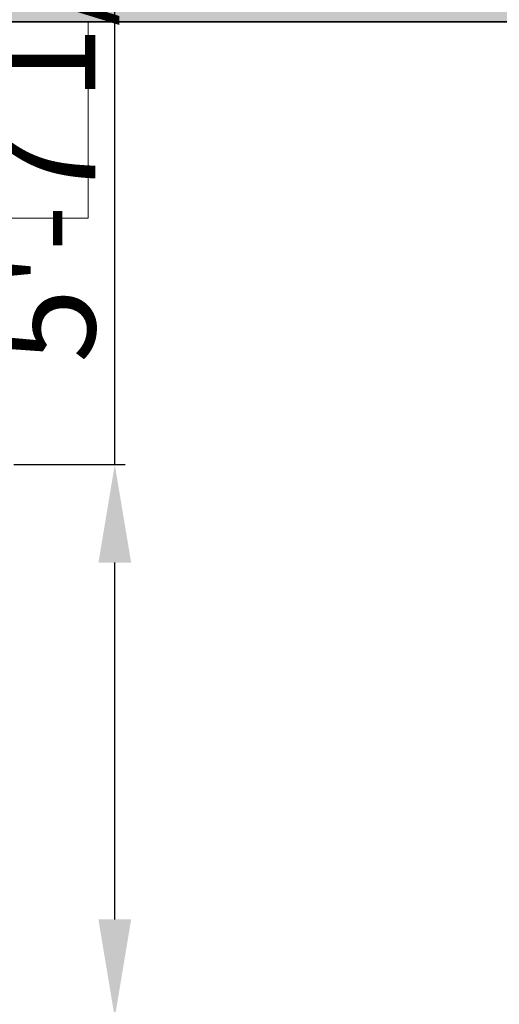
# Model space of a CAD drawing. Units: inches. Extents: x 2083 to 3317, y 1141 to 2115.
# Tile 14 of 256: x 2324 to 2382, y 1296 to 1417. Entities that reach past the tile are written whole.
import ezdxf

# ---------------------------------------------------------------- set-up
doc = ezdxf.new("R2010")
doc.units = ezdxf.units.IN
for name, color, linetype, lineweight in [('A-ANNO-DIMS', 2, 'Continuous', 18), ('A-FLOR-CASE', 8, 'Continuous', 18), ('A-WALL', 7, 'Continuous', 35)]:
    doc.layers.add(name, color=color, linetype=linetype, lineweight=lineweight)
doc.layers.add('A-WALL-PATT', color=251, linetype='Continuous', lineweight=13, true_color=0x636466)
doc.styles.get("Standard").update_dxf_attribs({"font": 'arial.ttf'})
doc.dimstyles.new('ISO-25', dxfattribs={"dimtxt": 12, "dimasz": 12, "dimexe": 1.25, "dimexo": 0.625, "dimtad": 1, "dimlunit": 3, "dimtxsty": 'Standard', "dimcen": 2.5, "dimadec": 0, "dimazin": 0, "dimtfac": 1, "dimtmove": 0, "dimatfit": 3, "dimfxl": 1, "dimarcsym": 0})

# ---------------------------------------------------------------- blocks, each defined once
blk = doc.blocks.new('CASEWORK-96X24')
for q in [(0, 0), (24, 96)]:
    blk.add_line((0, 96), q)
blk = doc.blocks.new('*D23')
at = {"layer": 'A-ANNO-DIMS', "color": 0, "lineweight": -2, "transparency": 16777216}
for p, q in [((2335.21, 1362.11), (2335.21, 1476.47)), ((2322.89, 1362.11), (2336.46, 1362.11)), ((2335.21, 1306.47), (2335.21, 1350.11)), ((2322.89, 1294.47), (2336.46, 1294.47))]:
    blk.add_line(p, q, dxfattribs=at)
at = {"layer": 'A-ANNO-DIMS', "color": 0, "transparency": 16777216}
for points in [[(2333.21, 1350.11), (2337.21, 1350.11), (2335.21, 1362.11)], [(2333.21, 1306.47), (2337.21, 1306.47), (2335.21, 1294.47)]]:
    blk.add_solid(points, dxfattribs=at)
at = {"layer": 'Defpoints', "color": 0, "transparency": 16777216}
for p in [(2322.26, 1362.11), (2335.21, 1362.11), (2322.26, 1294.47)]:
    blk.add_point(p, dxfattribs=at)
at = {"layer": 'A-ANNO-DIMS', "color": 0, "transparency": 16777216, "insert": (2328.38, 1425.29), "char_height": 12, "attachment_point": 5, "rotation": 90}
blk.add_mtext('5\'-7 1/2" TYP.', dxfattribs=at)
blk = doc.blocks.new('*D30')
at = {"layer": 'A-ANNO-DIMS', "color": 0, "lineweight": -2, "transparency": 16777216}
for p, q in [((2240.02, 1445.27), (2240.02, 1448.05)), ((2254.33, 1445.27), (2254.33, 1448.05)), ((2228.02, 1446.8), (2216.02, 1446.8)), ((2240.02, 1446.8), (2254.33, 1446.8)), ((2266.33, 1446.8), (2413.76, 1446.8))]:
    blk.add_line(p, q, dxfattribs=at)
at = {"layer": 'A-ANNO-DIMS', "color": 0, "transparency": 16777216}
for points in [[(2228.02, 1448.8), (2228.02, 1444.8), (2240.02, 1446.8)], [(2266.33, 1448.8), (2266.33, 1444.8), (2254.33, 1446.8)]]:
    blk.add_solid(points, dxfattribs=at)
at = {"layer": 'Defpoints', "color": 0, "transparency": 16777216}
for p in [(2254.33, 1446.8), (2240.02, 1444.65), (2254.33, 1444.65)]:
    blk.add_point(p, dxfattribs=at)
at = {"layer": 'A-ANNO-DIMS', "color": 0, "transparency": 16777216, "insert": (2346.05, 1453.63), "char_height": 12, "attachment_point": 5}
blk.add_mtext('WC 1\'-2 1/2" TYP.', dxfattribs=at)

msp = doc.modelspace()

# ---------------------------------------------------------------- hatches: boundary and pattern name
at = {"layer": 'A-WALL-PATT'}
h = msp.add_hatch(color=256, dxfattribs=at)
h.dxf.hatch_style = 1
h.paths.add_polyline_path([(3126.96, 2020.761), (2748.96, 2020.761), (2604.96, 2020.761), (2226.96, 2020.761), (2226.96, 1702.761), (2466.96, 1702.761), (2466.96, 1582.761), (2418.96, 1582.761), (2418.96, 1477.761), (2226.96, 1477.761), (2226.96, 1263.261), (2544.96, 1263.261), (2544.96, 1411.761), (2604.96, 1411.761), (2685.96, 1411.761), (2685.96, 1420.761), (2604.96, 1420.761), (2604.96, 1573.761), (2604.96, 1702.761), (2604.96, 2011.761), (2748.96, 2011.761), (2748.96, 1702.761), (2862.96, 1702.761), (2862.96, 1621.761), (2871.96, 1621.761), (2871.96, 1702.761), (2883.96, 1702.761), (2883.96, 1706.939, -0.0264593), (2883.96, 1711.761), (2757.96, 1711.761), (2757.96, 1807.761), (2787.96, 1807.761), (2787.96, 1812.261), (2757.96, 1812.261), (2757.96, 2011.761), (2877.96, 2011.761), (2877.96, 1812.261), (2847.96, 1812.261), (2847.96, 1807.761), (2889.836, 1807.761), (2889.836, 1812.261), (2882.46, 1812.261), (2882.46, 2011.761), (3117.96, 2011.761), (3117.96, 1812.261), (2937.836, 1812.261), (2937.836, 1807.761), (2995.71, 1807.761), (2995.71, 1796.118), (3000.21, 1796.118), (3000.21, 1807.761), (3117.96, 1807.761), (3117.96, 1711.761), (3000.21, 1711.761), (3000.21, 1760.118), (2998.573, 1760.118, -0.020711), (2995.71, 1760.118), (2995.71, 1711.761), (2931.96, 1711.761), (2931.96, 1702.761), (3126.96, 1702.761)])
h.paths.add_polyline_path([(2471.46, 2011.761), (2471.46, 1810.011), (2462.717, 1810.011), (2462.717, 1805.511), (2505.96, 1805.511), (2505.96, 1810.011), (2475.96, 1810.011), (2475.96, 2011.761), (2595.96, 2011.761), (2595.96, 1810.011), (2565.96, 1810.011), (2565.96, 1805.511), (2595.96, 1805.511), (2595.96, 1711.761), (2235.96, 1711.761), (2235.96, 1805.511), (2353.71, 1805.511), (2353.71, 1796.054), (2358.21, 1796.054), (2358.21, 1805.511), (2414.717, 1805.511), (2414.717, 1810.011), (2235.96, 1810.011), (2235.96, 2011.761)], flags=16)
h.paths.add_polyline_path([(2270.205, 1994.61), (2270.205, 1970.61), (2246.205, 1970.61), (2246.205, 1994.61)], flags=0)
edge = h.paths.add_edge_path(flags=0)
edge.add_ellipse((2332.027, 1899.798), major_axis=(-3.043, 3.043), ratio=0.1682525, start_angle=-161.33217, end_angle=-156.30711, ccw=False)
edge.add_ellipse((2333.082, 1898.744), major_axis=(-1.055, 1.055), ratio=0.4535321, start_angle=-123.37102, end_angle=-94.15911)
edge = h.paths.add_edge_path(flags=0)
edge.add_ellipse((2332.027, 1968.876), major_axis=(3.043, 3.043), ratio=0.1682525, start_angle=18.66783, end_angle=23.69289)
edge.add_spline(control_points=[(2332.926, 1970.691), (2332.227, 1970.336), (2330.894, 1969.659), (2328.413, 1970.932), (2327.204, 1967.749), (2324.71, 1969.956), (2322.533, 1967.012), (2320.013, 1971.296), (2317.68, 1968.158), (2316.041, 1967.102), (2315.427, 1966.81)], knot_values=[0, 0, 0, 0, 2.2670587, 4.3245589, 6.6855835, 8.8786411, 11.121502, 14.300359, 17.7552837, 19.732645, 19.732645, 19.732645, 19.732645], degree=3, periodic=0)
edge.add_ellipse((2332.027, 1968.876), major_axis=(3.043, 3.043), ratio=0.1682525, start_angle=18.66783, end_angle=23.69289, ccw=False)
edge.add_ellipse((2333.082, 1969.931), major_axis=(1.055, 1.055), ratio=0.4535321, start_angle=56.62898, end_angle=85.84089, ccw=False)
edge = h.paths.add_edge_path(flags=0)
edge.add_spline(control_points=[(2296.428, 1967.988), (2293.628, 1965.336), (2287.704, 1959.727), (2299.744, 1949.996), (2294.533, 1935.669), (2290.573, 1920.604), (2293.394, 1909.974), (2296.185, 1904.967)], knot_values=[0.0991853, 0.0991853, 0.0991853, 0.0991853, 0.3453009, 0.6198217, 0.9826526, 1.3860932, 1.8105546, 1.8105546, 1.8105546, 1.8105546], degree=3, periodic=0)
edge.add_spline(control_points=[(2296.185, 1904.967), (2297.384, 1902.619), (2298.001, 1901.949), (2298.553, 1901.468)], knot_values=[0.0062457, 0.0062457, 0.0062457, 0.0062457, 0.0554759, 0.0554759, 0.0554759, 0.0554759], degree=3, periodic=0)
edge.add_spline(control_points=[(2298.553, 1901.468), (2297.259, 1900.923), (2295.225, 1900.232), (2293.06, 1900.614), (2292.101, 1900.788), (2292.09, 1900.791)], knot_values=[0.3128349, 0.3128349, 0.3128349, 0.3128349, 0.4017797, 0.4749867, 0.4759027, 0.4759027, 0.4759027, 0.4759027], degree=3, periodic=0)
edge.add_arc((2292.794, 1904.664), 3.937, 215.4209, 259.69818, ccw=False)
edge.add_spline(control_points=[(2289.585, 1902.382), (2289.477, 1902.535), (2289.368, 1902.688), (2289.261, 1902.841)], knot_values=[0.1028719, 0.1028719, 0.1028719, 0.1028719, 0.1168958, 0.1168958, 0.1168958, 0.1168958], degree=3, periodic=0)
edge.add_spline(control_points=[(2289.261, 1902.841), (2288.687, 1902.55), (2287.64, 1902.02), (2285.881, 1901.874), (2283.853, 1901.504), (2281.72, 1899.711), (2278.467, 1899.493), (2276.157, 1901.883), (2272.259, 1899.804), (2267.778, 1901.843), (2262.244, 1900.184), (2257.415, 1901.782), (2254.318, 1900.726), (2253.178, 1900.337)], knot_values=[0, 0, 0, 0, 1.9079767, 3.4771759, 5.261074, 7.9728515, 11.6802485, 13.7179214, 16.9395917, 22.789562, 27.5025027, 33.5952153, 37.1456181, 37.1456181, 37.1456181, 37.1456181], degree=3, periodic=0)
edge.add_line((2253.178, 1900.337), (2250.244, 1902.841))
edge.add_line((2250.244, 1902.841), (2250.244, 1965.833))
edge.add_line((2250.244, 1965.833), (2253.178, 1968.337))
edge.add_spline(control_points=[(2253.178, 1968.337), (2254.318, 1967.948), (2257.415, 1966.892), (2262.244, 1968.49), (2267.778, 1966.831), (2271.527, 1968.537), (2273.876, 1967.828), (2274.207, 1967.728)], knot_values=[0, 0, 0, 0, 0.0901802, 0.2449351, 0.3646438, 0.5132331, 0.5378548, 0.5378548, 0.5378548, 0.5378548], degree=3, periodic=0)
edge.add_arc((2274.353, 1963.793), 3.937, 72.05113, 92.12795, ccw=False)
edge.add_arc((2281.297, 1985.23), 18.596, 252.05113, 288.56572)
edge.add_arc((2292.317, 1956.029), 12.646, 71.02679, 113.77822, ccw=False)
edge = h.paths.add_edge_path(flags=0)
edge.add_spline(control_points=[(2274.899, 1951.856), (2275.066, 1951.617), (2275.233, 1951.377), (2275.398, 1951.136)], knot_values=[1.4099157, 1.4099157, 1.4099157, 1.4099157, 1.4315903, 1.4315903, 1.4315903, 1.4315903], degree=3, periodic=0)
edge.add_spline(control_points=[(2275.398, 1951.136), (2275.792, 1950.562), (2276.179, 1949.984), (2276.546, 1949.397)], knot_values=[1.3582378, 1.3582378, 1.3582378, 1.3582378, 1.4099157, 1.4099157, 1.4099157, 1.4099157], degree=3, periodic=0)
edge.add_line((2276.546, 1949.397), (2277.437, 1947.862))
edge.add_spline(control_points=[(2277.437, 1947.862), (2276.304, 1945.673), (2274.64, 1942.427), (2274.632, 1938.094), (2272.799, 1930.852), (2274.356, 1943.897), (2275.948, 1947.923), (2276.546, 1949.397)], knot_values=[0.0056315, 0.0056315, 0.0056315, 0.0056315, 0.1860139, 0.2660015, 0.3570872, 0.5963902, 0.7397317, 0.7397317, 0.7397317, 0.7397317], degree=3, periodic=0)
edge.add_spline(control_points=[(2276.546, 1949.397), (2276.179, 1949.984), (2275.792, 1950.562), (2275.398, 1951.136)], knot_values=[1.3582378, 1.3582378, 1.3582378, 1.3582378, 1.4099157, 1.4099157, 1.4099157, 1.4099157], degree=3, periodic=0)
edge.add_spline(control_points=[(2275.398, 1951.136), (2274.943, 1950.08), (2274.208, 1948.025), (2273.935, 1944.851), (2272.469, 1937.627), (2273.466, 1945.696), (2274.701, 1951.059), (2274.899, 1951.856)], knot_values=[0.1043639, 0.1043639, 0.1043639, 0.1043639, 0.1896363, 0.2696239, 0.3607096, 0.6000126, 0.6446217, 0.6446217, 0.6446217, 0.6446217], degree=3, periodic=0)
h.paths.add_polyline_path([(2269.168, 1963.128, -0.3575267), (2268.171, 1960.976, -0.0925607), (2268.171, 1939.436, -0.3575267), (2269.168, 1937.285, -0.3575267), (2267.016, 1938.282, -0.1647847), (2254.686, 1938.282, -0.3575267), (2252.534, 1937.285, -0.3575267), (2253.531, 1939.436, -0.0925607), (2253.531, 1960.976, -0.3575267), (2252.534, 1963.128, -0.3575267), (2254.686, 1962.131, -0.1647847), (2267.016, 1962.131, -0.3575267)], flags=0)
h.paths.add_polyline_path([(2248.874, 1967.802), (2248.874, 1957.028), (2249.458, 1957.028), (2249.458, 1911.647), (2248.874, 1911.647), (2248.874, 1900.873), (2246.512, 1900.873, 0.1973271), (2244.15, 1902.457), (2244.15, 1966.218, 0.1973271), (2246.512, 1967.802)], flags=0)
h.paths.add_polyline_path([(2269.168, 1931.389, -0.3575267), (2268.171, 1929.238, -0.0925607), (2268.171, 1907.698, -0.3575267), (2269.168, 1905.547, -0.3575267), (2267.016, 1906.544, -0.1647847), (2254.686, 1906.544, -0.3575267), (2252.534, 1905.547, -0.3575267), (2253.531, 1907.698, -0.0925607), (2253.531, 1929.238, -0.3575267), (2252.534, 1931.389, -0.3575267), (2254.686, 1930.392, -0.1647847), (2267.016, 1930.392, -0.3575267)], flags=0)
edge = h.paths.add_edge_path(flags=0)
edge.add_spline(control_points=[(2276.197, 1906.724), (2276.168, 1909.029), (2276.114, 1913.372), (2270.598, 1924.925), (2273.905, 1919.013), (2275.922, 1916.262), (2275.475, 1912.402), (2277.258, 1910.381), (2276.696, 1908.225), (2276.646, 1906.813), (2276.618, 1906.008)], knot_values=[0, 0, 0, 0, 8.6102597, 16.2212739, 18.8430575, 23.8048978, 27.4408283, 29.3561016, 31.2034776, 33.6506866, 33.6506866, 33.6506866, 33.6506866], degree=3, periodic=0)
edge.add_spline(control_points=[(2276.618, 1906.008), (2276.623, 1905.624), (2276.498, 1904.629), (2275.442, 1903.855), (2274.937, 1903.08), (2274.859, 1902.841)], knot_values=[0.1564884, 0.1564884, 0.1564884, 0.1564884, 0.1843975, 0.2313765, 0.2505985, 0.2505985, 0.2505985, 0.2505985], degree=3, periodic=0)
edge.add_line((2274.859, 1902.841), (2276.506, 1902.841))
edge.add_spline(control_points=[(2276.506, 1902.841), (2276.788, 1903.085), (2277.665, 1904.125), (2278.25, 1904.341), (2277.654, 1908.527), (2278.156, 1906.228), (2278.1, 1905.286), (2278.847, 1904.069), (2277.857, 1903.415), (2277.874, 1902.991), (2277.904, 1902.841)], knot_values=[0.0595743, 0.0595743, 0.0595743, 0.0595743, 0.0807529, 0.1037415, 0.1697201, 0.1760361, 0.2071372, 0.2404744, 0.2623409, 0.2736605, 0.2736605, 0.2736605, 0.2736605], degree=3, periodic=0)
edge.add_line((2277.904, 1902.841), (2280.03, 1902.841))
edge.add_spline(control_points=[(2280.03, 1902.841), (2279.888, 1903.088), (2279.499, 1903.982), (2280.152, 1905.939), (2278.104, 1909.658), (2279.762, 1907.185), (2280.328, 1904.875), (2280.485, 1903.49), (2281.463, 1903.249), (2281.758, 1902.936), (2281.834, 1902.841)], knot_values=[0.013856, 0.013856, 0.013856, 0.013856, 0.0348738, 0.0888667, 0.1078792, 0.1267378, 0.158714, 0.1937575, 0.2174868, 0.2267221, 0.2267221, 0.2267221, 0.2267221], degree=3, periodic=0)
edge.add_spline(control_points=[(2281.834, 1902.841), (2281.788, 1902.827), (2281.647, 1902.783), (2281.396, 1902.859), (2281.088, 1902.985), (2280.721, 1903.061), (2280.333, 1903.026), (2280.125, 1902.899), (2280.03, 1902.841)], knot_values=[0, 0, 0, 0, 0.1441304, 0.435517, 0.7492759, 1.1530457, 1.5483707, 1.878348, 1.878348, 1.878348, 1.878348], degree=3, periodic=0)
edge.add_line((2280.03, 1902.841), (2277.904, 1902.841))
edge.add_spline(control_points=[(2277.904, 1902.841), (2277.893, 1902.796), (2277.865, 1902.68), (2277.607, 1902.687), (2277.274, 1902.801), (2276.838, 1902.62), (2276.584, 1902.789), (2276.506, 1902.841)], knot_values=[0, 0, 0, 0, 0.1271885, 0.3261988, 0.6280094, 1.2435704, 1.5153306, 1.5153306, 1.5153306, 1.5153306], degree=3, periodic=0)
edge.add_line((2276.506, 1902.841), (2274.859, 1902.841))
edge.add_spline(control_points=[(2274.859, 1902.841), (2274.814, 1902.899), (2274.725, 1903.013), (2274.493, 1903.119), (2274.244, 1902.961), (2273.937, 1903.185), (2273.614, 1902.983), (2273.408, 1902.883), (2273.322, 1902.841)], knot_values=[0, 0, 0, 0, 0.2184302, 0.4369566, 0.6879766, 0.9903786, 1.3983955, 1.6918498, 1.6918498, 1.6918498, 1.6918498], degree=3, periodic=0)
edge.add_spline(control_points=[(2273.322, 1902.841), (2273.617, 1903.446), (2274.274, 1904.538), (2276.027, 1904.574), (2276.207, 1906.584), (2276.197, 1906.724)], knot_values=[0.0122268, 0.0122268, 0.0122268, 0.0122268, 0.0594721, 0.1062177, 0.134458, 0.134458, 0.134458, 0.134458], degree=3, periodic=0)
h.paths.add_polyline_path([(2270.776, 1897.79), (2270.776, 1873.79), (2246.776, 1873.79), (2246.776, 1897.79)], flags=0)
h.paths.add_polyline_path([(2353.71, 1760.005), (2353.71, 1760.054), (2358.21, 1760.054, -0.033729)], flags=0)
h.paths.add_polyline_path([(2321.819, 1737.529), (2341.995, 1737.529, -0.4142136), (2343.203, 1736.321), (2343.203, 1721.021, -0.4142136), (2341.995, 1719.813), (2321.819, 1719.813, -0.4142136), (2320.611, 1721.021), (2320.611, 1736.321, -0.4142136)], flags=0)
h.paths.add_polyline_path([(2324.235, 1736.321), (2339.579, 1736.321, -0.4142136), (2341.995, 1733.905), (2341.995, 1725.45, -0.4142136), (2339.579, 1723.034), (2333.681, 1723.034), (2333.845, 1722.045, -0.8706461), (2335.425, 1721.826, -0.767327), (2333.923, 1721.423), (2331.291, 1721.423, -0.767327), (2329.788, 1721.826, -0.8706461), (2331.368, 1722.045), (2331.533, 1723.034), (2324.235, 1723.034, -0.4142136), (2321.819, 1725.45), (2321.819, 1733.905, -0.4142136)], flags=0)
h.paths.add_polyline_path([(2570.484, 1928.615), (2589.684, 1928.615), (2590.169, 1928.615), (2590.169, 1904.993), (2570.484, 1904.993)], flags=0)
h.paths.add_polyline_path([(2574.447, 1927.264, -1), (2572.829, 1927.264, -1)], flags=0)
h.paths.add_polyline_path([(2573.09, 1926.941), (2573.925, 1927.776), (2574.148, 1927.553), (2573.313, 1926.718)], flags=0)
h.paths.add_polyline_path([(2578.779, 1919.73, -1), (2571.592, 1919.73, -1)], flags=0)
h.paths.add_polyline_path([(2578.385, 1919.73, -1), (2571.985, 1919.73, -1)], flags=0)
h.paths.add_polyline_path([(2331.596, 1729.476, -1), (2333.618, 1729.476, -1)], flags=0)
h.paths.add_polyline_path([(2578.034, 1927.264, -1), (2576.416, 1927.264, -1)], flags=0)
h.paths.add_polyline_path([(2576.689, 1927.531), (2576.912, 1927.754), (2577.747, 1926.919), (2577.524, 1926.696)], flags=0)
h.paths.add_polyline_path([(2578.139, 1909.86, -1), (2572.232, 1909.86, -1)], flags=0)
h.paths.add_polyline_path([(2577.745, 1909.86, -1), (2572.625, 1909.86, -1)], flags=0)
h.paths.add_polyline_path([(2583.798, 1927.264, -1), (2582.179, 1927.264, -1)], flags=0)
h.paths.add_polyline_path([(2582.719, 1927.754), (2583.554, 1926.919), (2583.331, 1926.696), (2582.496, 1927.531)], flags=0)
h.paths.add_polyline_path([(2582.496, 1927.531), (2582.719, 1927.754), (2583.554, 1926.919), (2583.331, 1926.696)], flags=0)
h.paths.add_polyline_path([(2587.739, 1920.53, -1), (2581.832, 1920.53, -1)], flags=0)
h.paths.add_polyline_path([(2587.345, 1920.53, -1), (2582.225, 1920.53, -1)], flags=0)
h.paths.add_polyline_path([(2587.385, 1927.264, -1), (2585.766, 1927.264, -1)], flags=0)
h.paths.add_polyline_path([(2586.082, 1926.98), (2586.917, 1927.815), (2587.14, 1927.593), (2586.305, 1926.758)], flags=0)
h.paths.add_polyline_path([(2588.379, 1910.66, -1), (2581.192, 1910.66, -1)], flags=0)
h.paths.add_polyline_path([(2587.985, 1910.66, -1), (2581.585, 1910.66, -1)], flags=0)
h.paths.add_polyline_path([(2417.168, 1729.478), (2437.344, 1729.478, -0.4142136), (2438.552, 1728.27), (2438.552, 1712.969, -0.4142136), (2437.344, 1711.761), (2417.168, 1711.761, -0.4142136), (2415.96, 1712.969), (2415.96, 1728.27, -0.4142136)], flags=0)
h.paths.add_polyline_path([(2419.584, 1728.27), (2434.928, 1728.27, -0.4142136), (2437.344, 1725.854), (2437.344, 1717.398, -0.4142136), (2434.928, 1714.983), (2429.029, 1714.983), (2429.194, 1713.994, -0.8706461), (2430.774, 1713.775, -0.767327), (2429.271, 1713.372), (2426.64, 1713.372, -0.767327), (2425.137, 1713.775, -0.8706461), (2426.717, 1713.994), (2426.882, 1714.983), (2419.584, 1714.983, -0.4142136), (2417.168, 1717.398), (2417.168, 1725.854, -0.4142136)], flags=0)
h.paths.add_polyline_path([(2419.584, 1728.27), (2434.928, 1728.27, -0.4142136), (2437.344, 1725.854), (2437.344, 1717.398, -0.4142136), (2434.928, 1714.983), (2429.029, 1714.983), (2428.358, 1719.009), (2427.553, 1719.009), (2426.882, 1714.983), (2419.584, 1714.983, -0.4142136), (2417.168, 1717.398), (2417.168, 1725.854, -0.4142136)], flags=0)
h.paths.add_polyline_path([(2426.944, 1721.425, -1), (2428.967, 1721.425, -1)], flags=0)
h.paths.add_polyline_path([(2475.96, 1702.761), (2595.96, 1702.761), (2595.96, 1582.761), (2475.96, 1582.761)], flags=16)
h.paths.add_polyline_path([(2427.96, 1573.761), (2595.96, 1573.761), (2595.96, 1468.761), (2595.96, 1420.761), (2384.46, 1420.761), (2384.46, 1468.761), (2427.96, 1468.761)], flags=16)
h.paths.add_polyline_path([(2379.96, 1468.761), (2379.96, 1420.761), (2235.96, 1420.761), (2235.96, 1468.761)], flags=16)
h.paths.add_polyline_path([(2317.816, 1466.696), (2337.992, 1466.696, -0.4142136), (2339.2, 1465.488), (2339.2, 1450.187, -0.4142136), (2337.992, 1448.979), (2317.816, 1448.979, -0.4142136), (2316.608, 1450.187), (2316.608, 1465.488, -0.4142136)], flags=0)
h.paths.add_polyline_path([(2320.232, 1465.488), (2335.576, 1465.488, -0.4142136), (2337.992, 1463.072), (2337.992, 1454.616, -0.4142136), (2335.576, 1452.2), (2329.677, 1452.2), (2329.842, 1451.212, -0.8706461), (2331.422, 1450.992, -0.767327), (2329.92, 1450.59), (2327.288, 1450.59, -0.767327), (2325.785, 1450.992, -0.8706461), (2327.365, 1451.212), (2327.53, 1452.2), (2320.232, 1452.2, -0.4142136), (2317.816, 1454.616), (2317.816, 1463.072, -0.4142136)], flags=0)
h.paths.add_polyline_path([(2320.232, 1465.488), (2335.576, 1465.488, -0.4142136), (2337.992, 1463.072), (2337.992, 1454.616, -0.4142136), (2335.576, 1452.2), (2329.677, 1452.2), (2329.006, 1456.227), (2328.201, 1456.227), (2327.53, 1452.2), (2320.232, 1452.2, -0.4142136), (2317.816, 1454.616), (2317.816, 1463.072, -0.4142136)], flags=0)
h.paths.add_polyline_path([(2327.593, 1458.643, -1), (2329.615, 1458.643, -1)], flags=0)
h.paths.add_polyline_path([(2244.412, 1433.34), (2241.921, 1433.34, -0.4142136), (2240.018, 1435.244), (2240.018, 1440.953, -0.4142105), (2241.921, 1442.856), (2244.412, 1442.856, -1.9764724)], flags=0)
h.paths.add_polyline_path([(2245.357, 1434.398, -0.4142136), (2245.357, 1441.799, -2.1440985)], flags=0)
h.paths.add_polyline_path([(2535.96, 1416.261), (2535.96, 1272.261), (2235.96, 1272.261), (2235.96, 1416.261)], flags=16)
h.paths.add_polyline_path([(2260.12, 1384.293), (2260.12, 1362.039), (2237.865, 1362.039), (2237.865, 1384.293)], flags=0)
edge = h.paths.add_edge_path(flags=0)
edge.add_line((2318.252, 1362.093), (2318.146, 1362.001))
edge.add_ellipse((2317.445, 1360.431), major_axis=(2.822, 2.822), ratio=0.1682525, start_angle=18.66783, end_angle=20.94813, ccw=False)
edge.add_ellipse((2318.423, 1361.409), major_axis=(0.978, 0.978), ratio=0.4535321, start_angle=56.62898, end_angle=70.2262, ccw=False)
edge = h.paths.add_edge_path(flags=0)
edge.add_line((2319.107, 1295.571), (2319.015, 1295.677))
edge.add_ellipse((2317.445, 1296.378), major_axis=(-2.822, 2.822), ratio=0.1682525, start_angle=-161.33217, end_angle=-159.05187, ccw=False)
edge.add_ellipse((2318.423, 1295.4), major_axis=(-0.978, 0.978), ratio=0.4535321, start_angle=-123.37102, end_angle=-109.7738)
edge = h.paths.add_edge_path(flags=0)
edge.add_spline(control_points=[(2284.21, 1301.17), (2284.581, 1300.445), (2284.891, 1299.892), (2285.16, 1299.461)], knot_values=[0.0390658, 0.0390658, 0.0390658, 0.0390658, 0.0554759, 0.0554759, 0.0554759, 0.0554759], degree=3, periodic=0)
edge.add_line((2285.16, 1299.461), (2284.21, 1301.17))
edge = h.paths.add_edge_path(flags=0)
edge.add_line((2280.412, 1297.298), (2283.37, 1297.036))
edge.add_line((2283.37, 1297.036), (2286.406, 1297.926))
edge.add_spline(control_points=[(2286.406, 1297.926), (2285.305, 1297.463), (2284.345, 1297.129), (2283.37, 1297.036)], knot_values=[0.3943688, 0.3943688, 0.3943688, 0.3943688, 0.4759027, 0.4759027, 0.4759027, 0.4759027], degree=3, periodic=0)
edge.add_spline(control_points=[(2283.37, 1297.036), (2283.281, 1297.028), (2282.316, 1296.957), (2281.313, 1297.134), (2280.423, 1297.296), (2280.412, 1297.298)], knot_values=[0.3128349, 0.3128349, 0.3128349, 0.3128349, 0.3202458, 0.3934528, 0.3943688, 0.3943688, 0.3943688, 0.3943688], degree=3, periodic=0)
edge = h.paths.add_edge_path(flags=0)
edge.add_line((2284.436, 1359.607), (2280.446, 1355.328))
edge.add_line((2280.446, 1355.328), (2279.58, 1351.018))
edge.add_line((2279.58, 1351.018), (2282.413, 1346.58))
edge.add_spline(control_points=[(2282.413, 1346.58), (2283.153, 1345.589), (2284.253, 1344.029), (2284.801, 1342.387), (2284.935, 1341.806)], knot_values=[1.2400982, 1.2400982, 1.2400982, 1.2400982, 1.3328922, 1.3827123, 1.3827123, 1.3827123, 1.3827123], degree=3, periodic=0)
edge.add_spline(control_points=[(2284.935, 1341.806), (2285.319, 1340.141), (2285.233, 1338.409), (2284.91, 1336.654)], knot_values=[1.0974841, 1.0974841, 1.0974841, 1.0974841, 1.2400982, 1.2400982, 1.2400982, 1.2400982], degree=3, periodic=0)
edge.add_spline(control_points=[(2284.91, 1336.654), (2284.587, 1334.899), (2284.027, 1333.12), (2283.463, 1331.361)], knot_values=[0.9548699, 0.9548699, 0.9548699, 0.9548699, 1.0974841, 1.0974841, 1.0974841, 1.0974841], degree=3, periodic=0)
edge.add_line((2283.463, 1331.361), (2281.89, 1326.153))
edge.add_line((2281.89, 1326.153), (2280.756, 1321.056))
edge.add_line((2280.756, 1321.056), (2280.299, 1316.002))
edge.add_line((2280.299, 1316.002), (2280.716, 1310.95))
edge.add_line((2280.716, 1310.95), (2282.028, 1305.972))
edge.add_line((2282.028, 1305.972), (2284.21, 1301.17))
edge.add_spline(control_points=[(2284.21, 1301.17), (2283.341, 1302.73), (2282.612, 1304.336), (2282.028, 1305.972)], knot_values=[0.0991853, 0.0991853, 0.0991853, 0.0991853, 0.2417994, 0.2417994, 0.2417994, 0.2417994], degree=3, periodic=0)
edge.add_spline(control_points=[(2282.028, 1305.972), (2281.444, 1307.608), (2281.005, 1309.273), (2280.716, 1310.95)], knot_values=[0.2417994, 0.2417994, 0.2417994, 0.2417994, 0.3844135, 0.3844135, 0.3844135, 0.3844135], degree=3, periodic=0)
edge.add_spline(control_points=[(2280.716, 1310.95), (2280.433, 1312.588), (2280.289, 1314.277), (2280.299, 1315.962), (2280.299, 1316.002)], knot_values=[0.3844135, 0.3844135, 0.3844135, 0.3844135, 0.5236467, 0.5270276, 0.5270276, 0.5270276, 0.5270276], degree=3, periodic=0)
edge.add_spline(control_points=[(2280.299, 1316.002), (2280.312, 1317.687), (2280.478, 1319.368), (2280.756, 1321.056)], knot_values=[0.5270276, 0.5270276, 0.5270276, 0.5270276, 0.6696417, 0.6696417, 0.6696417, 0.6696417], degree=3, periodic=0)
edge.add_spline(control_points=[(2280.756, 1321.056), (2281.035, 1322.744), (2281.426, 1324.44), (2281.89, 1326.153)], knot_values=[0.6696417, 0.6696417, 0.6696417, 0.6696417, 0.8122558, 0.8122558, 0.8122558, 0.8122558], degree=3, periodic=0)
edge.add_spline(control_points=[(2281.89, 1326.153), (2282.264, 1327.533), (2282.788, 1329.262), (2283.353, 1331.018), (2283.463, 1331.361)], knot_values=[0.8122558, 0.8122558, 0.8122558, 0.8122558, 0.9270873, 0.9548699, 0.9548699, 0.9548699, 0.9548699], degree=3, periodic=0)
edge.add_line((2283.463, 1331.361), (2284.91, 1336.654))
edge.add_line((2284.91, 1336.654), (2284.935, 1341.806))
edge.add_line((2284.935, 1341.806), (2282.413, 1346.58))
edge.add_spline(control_points=[(2282.413, 1346.58), (2281.275, 1348.104), (2280.078, 1349.57), (2279.58, 1351.018)], knot_values=[1.3827123, 1.3827123, 1.3827123, 1.3827123, 1.5253264, 1.5253264, 1.5253264, 1.5253264], degree=3, periodic=0)
edge.add_spline(control_points=[(2279.58, 1351.018), (2279.443, 1351.415), (2279.136, 1352.857), (2279.735, 1354.29), (2280.446, 1355.328)], knot_values=[1.5253264, 1.5253264, 1.5253264, 1.5253264, 1.564439, 1.6679405, 1.6679405, 1.6679405, 1.6679405], degree=3, periodic=0)
edge.add_spline(control_points=[(2280.446, 1355.328), (2281.426, 1356.758), (2282.931, 1358.183), (2284.436, 1359.607)], knot_values=[1.6679405, 1.6679405, 1.6679405, 1.6679405, 1.8105546, 1.8105546, 1.8105546, 1.8105546], degree=3, periodic=0)
edge.add_arc((2280.623, 1348.518), 11.726, 71.02679, 113.77822)
edge.add_arc((2270.405, 1375.595), 17.244, 252.05113, 288.56572, ccw=False)
edge.add_arc((2263.966, 1355.718), 3.651, 72.05113, 92.12795)
edge.add_arc((2263.966, 1355.718), 3.651, 92.12795, 177.98513)
edge.add_spline(control_points=[(2260.318, 1355.846), (2260.26, 1354.221), (2260.551, 1350.187), (2262.999, 1346.766), (2264.473, 1344.649)], knot_values=[1.4315903, 1.4315903, 1.4315903, 1.4315903, 1.5641438, 1.7706953, 1.7706953, 1.7706953, 1.7706953], degree=3, periodic=0)
edge.add_line((2264.473, 1344.649), (2264.936, 1343.983))
edge.add_spline(control_points=[(2263.801, 1340.248), (2263.843, 1340.514), (2264.067, 1341.756), (2264.513, 1343.002), (2264.935, 1343.981)], knot_values=[0.5365702, 0.5365702, 0.5365702, 0.5365702, 0.5593494, 0.6446217, 0.6446217, 0.6446217, 0.6446217], degree=3, periodic=0)
edge.add_spline(control_points=[(2264.935, 1343.981), (2265.118, 1343.715), (2265.299, 1343.448), (2265.477, 1343.179)], knot_values=[1.3840767, 1.3840767, 1.3840767, 1.3840767, 1.4099157, 1.4099157, 1.4099157, 1.4099157], degree=3, periodic=0)
edge.add_spline(control_points=[(2265.477, 1343.179), (2265.655, 1342.911), (2265.829, 1342.641), (2265.999, 1342.369)], knot_values=[1.3582378, 1.3582378, 1.3582378, 1.3582378, 1.3840767, 1.3840767, 1.3840767, 1.3840767], degree=3, periodic=0)
edge.add_line((2265.999, 1342.369), (2266.826, 1340.946))
edge.add_spline(control_points=[(2266.826, 1340.946), (2268.894, 1337.09), (2271.398, 1325.843), (2270.516, 1310.569), (2275.919, 1301.861), (2277.79, 1299.199)], knot_values=[0.1168958, 0.1168958, 0.1168958, 0.1168958, 0.4729873, 1.0509689, 1.3137934, 1.3137934, 1.3137934, 1.3137934], degree=3, periodic=0)
edge.add_spline(control_points=[(2277.79, 1299.199), (2277.839, 1299.128), (2277.889, 1299.057), (2277.94, 1298.987)], knot_values=[0.1098839, 0.1098839, 0.1098839, 0.1098839, 0.1168958, 0.1168958, 0.1168958, 0.1168958], degree=3, periodic=0)
edge.add_line((2277.94, 1298.987), (2277.789, 1299.199))
edge.add_spline(control_points=[(2277.789, 1299.199), (2277.257, 1298.929), (2276.286, 1298.438), (2275.039, 1298.334), (2274.383, 1298.239), (2274.215, 1298.209)], knot_values=[33.1218702, 33.1218702, 33.1218702, 33.1218702, 35.0290557, 36.5982549, 37.1448269, 37.1448269, 37.1448269, 37.1448269], degree=3, periodic=0)
edge.add_line((2274.215, 1298.209), (2273.073, 1297.893))
edge.add_spline(control_points=[(2273.073, 1297.893), (2272.323, 1297.58), (2271.039, 1296.511), (2269.248, 1296.226), (2268.423, 1296.375)], knot_values=[26.5325843, 26.5325843, 26.5325843, 26.5325843, 29.198919, 31.8391012, 31.8391012, 31.8391012, 31.8391012], degree=3, periodic=0)
edge.add_line((2268.423, 1296.375), (2263.879, 1297.458))
edge.add_spline(control_points=[(2263.879, 1297.458), (2263.556, 1297.359), (2261.86, 1296.839), (2260.239, 1297.282), (2258.933, 1297.516)], knot_values=[15.9195506, 15.9195506, 15.9195506, 15.9195506, 16.9395917, 21.2260675, 21.2260675, 21.2260675, 21.2260675], degree=3, periodic=0)
edge.add_line((2258.933, 1297.516), (2254.055, 1297.329))
edge.add_spline(control_points=[(2254.055, 1297.329), (2253.756, 1297.296), (2252.114, 1297.165), (2250.462, 1297.544), (2249.13, 1297.668)], knot_values=[5.3065169, 5.3065169, 5.3065169, 5.3065169, 6.2764352, 10.6130337, 10.6130337, 10.6130337, 10.6130337], degree=3, periodic=0)
edge.add_line((2249.13, 1297.668), (2244.332, 1296.878))
edge.add_line((2244.332, 1296.878), (2241.611, 1299.199))
edge.add_line((2241.611, 1299.199), (2241.611, 1357.609))
edge.add_line((2241.611, 1357.609), (2244.332, 1359.931))
edge.add_line((2244.332, 1359.931), (2252.729, 1359.543))
edge.add_spline(control_points=[(2252.729, 1359.543), (2252.871, 1359.546), (2253.306, 1359.548), (2253.74, 1359.514), (2254.032, 1359.482)], knot_values=[0.233291, 0.233291, 0.233291, 0.233291, 0.2449351, 0.2689274, 0.2689274, 0.2689274, 0.2689274], degree=3, periodic=0)
edge.add_line((2254.032, 1359.482), (2259.587, 1359.416))
edge.add_spline(control_points=[(2259.587, 1359.416), (2260.677, 1359.629), (2262.073, 1359.897), (2263.524, 1359.459), (2263.83, 1359.366)], knot_values=[0.4225164, 0.4225164, 0.4225164, 0.4225164, 0.5132331, 0.5378548, 0.5378548, 0.5378548, 0.5378548], degree=3, periodic=0)
edge.add_arc((2263.966, 1355.718), 3.651, 72.05113, 92.12795, ccw=False)
edge.add_arc((2270.405, 1375.595), 17.244, 252.05113, 288.56572)
edge.add_arc((2280.623, 1348.518), 11.726, 71.02679, 113.77822, ccw=False)
h.paths.add_polyline_path([(2240.341, 1359.435), (2240.341, 1349.444), (2240.882, 1349.444), (2240.882, 1307.365), (2240.341, 1307.365), (2240.341, 1297.374), (2238.15, 1297.374, 0.1973271), (2235.96, 1298.843), (2235.96, 1357.966, 0.1973271), (2238.15, 1359.435)], flags=0)
h.paths.add_polyline_path([(2259.158, 1355.101, -0.3575267), (2258.233, 1353.106, -0.0925607), (2258.233, 1333.133, -0.3575267), (2259.158, 1331.138, -0.3575267), (2257.163, 1332.062, -0.1647847), (2245.729, 1332.062, -0.3575267), (2243.735, 1331.138, -0.3575267), (2244.659, 1333.133, -0.0925607), (2244.659, 1353.106, -0.3575267), (2243.735, 1355.101, -0.3575267), (2245.729, 1354.176, -0.1647847), (2257.163, 1354.176, -0.3575267)], flags=0)
edge = h.paths.add_edge_path(flags=0)
edge.add_line((2265.999, 1342.369), (2266.826, 1340.946))
edge.add_line((2266.826, 1340.946), (2265.308, 1337.814))
edge.add_line((2265.308, 1337.814), (2264.358, 1334.653))
edge.add_line((2264.358, 1334.653), (2264.262, 1333.8))
edge.add_spline(control_points=[(2264.262, 1333.8), (2264.208, 1333.187), (2264.162, 1332.366), (2264.007, 1331.414), (2263.969, 1331.202)], knot_values=[0.4644442, 0.4644442, 0.4644442, 0.4644442, 0.5166905, 0.5316081, 0.5316081, 0.5316081, 0.5316081], degree=3, periodic=0)
edge.add_spline(control_points=[(2263.969, 1331.202), (2263.775, 1330.119), (2263.424, 1328.791), (2263.257, 1328.531), (2263.234, 1328.515)], knot_values=[0.3726816, 0.3726816, 0.3726816, 0.3726816, 0.4488497, 0.4644442, 0.4644442, 0.4644442, 0.4644442], degree=3, periodic=0)
edge.add_spline(control_points=[(2263.234, 1328.515), (2263.096, 1328.42), (2263.131, 1329.301), (2263.275, 1330.616)], knot_values=[0.2809191, 0.2809191, 0.2809191, 0.2809191, 0.3726816, 0.3726816, 0.3726816, 0.3726816], degree=3, periodic=0)
edge.add_spline(control_points=[(2263.275, 1330.616), (2263.419, 1331.93), (2263.672, 1333.677), (2263.97, 1335.315)], knot_values=[0.1891566, 0.1891566, 0.1891566, 0.1891566, 0.2809191, 0.2809191, 0.2809191, 0.2809191], degree=3, periodic=0)
edge.add_spline(control_points=[(2263.97, 1335.315), (2264.1, 1336.032), (2264.419, 1337.622), (2264.755, 1338.864), (2264.947, 1339.491)], knot_values=[0.097394, 0.097394, 0.097394, 0.097394, 0.1375775, 0.1891566, 0.1891566, 0.1891566, 0.1891566], degree=3, periodic=0)
edge.add_spline(control_points=[(2264.947, 1339.491), (2265.29, 1340.606), (2265.644, 1341.494), (2265.999, 1342.369)], knot_values=[0.0056315, 0.0056315, 0.0056315, 0.0056315, 0.097394, 0.097394, 0.097394, 0.097394], degree=3, periodic=0)
h.paths.add_polyline_path([(2259.158, 1325.671, -0.3575267), (2258.233, 1323.676, -0.0925607), (2258.233, 1303.703, -0.3575267), (2259.158, 1301.708, -0.3575267), (2257.163, 1302.633, -0.1647847), (2245.729, 1302.633, -0.3575267), (2243.735, 1301.708, -0.3575267), (2244.659, 1303.703, -0.0925607), (2244.659, 1323.676, -0.3575267), (2243.735, 1325.671, -0.3575267), (2245.729, 1324.747, -0.1647847), (2257.163, 1324.747, -0.3575267)], flags=0)
edge = h.paths.add_edge_path(flags=0)
edge.add_spline(control_points=[(2261.709, 1317.311), (2261.679, 1317.418), (2261.762, 1317.389), (2262.491, 1316.09), (2262.962, 1315.301)], knot_values=[14.9558607, 14.9558607, 14.9558607, 14.9558607, 16.2212739, 18.6948259, 18.6948259, 18.6948259, 18.6948259], degree=3, periodic=0)
edge.add_spline(control_points=[(2262.962, 1315.301), (2262.99, 1315.254), (2263.702, 1314.067), (2264.349, 1313.127), (2264.73, 1312.164)], knot_values=[18.6948259, 18.6948259, 18.6948259, 18.6948259, 18.8430575, 22.433791, 22.433791, 22.433791, 22.433791], degree=3, periodic=0)
edge.add_spline(control_points=[(2264.73, 1312.164), (2264.876, 1311.796), (2265.177, 1310.77), (2265.143, 1309.559), (2265.248, 1308.824)], knot_values=[22.433791, 22.433791, 22.433791, 22.433791, 23.8048978, 26.1727562, 26.1727562, 26.1727562, 26.1727562], degree=3, periodic=0)
edge.add_line((2265.248, 1308.824), (2265.851, 1307.172))
edge.add_spline(control_points=[(2265.851, 1307.172), (2266.065, 1306.822), (2266.384, 1306.332), (2266.424, 1305.781), (2266.42, 1305.611)], knot_values=[28.0625624, 28.0625624, 28.0625624, 28.0625624, 29.3561016, 29.9117214, 29.9117214, 29.9117214, 29.9117214], degree=3, periodic=0)
edge.add_spline(control_points=[(2266.42, 1305.611), (2266.416, 1305.433), (2266.394, 1305.25), (2266.365, 1305.066)], knot_values=[29.9117214, 29.9117214, 29.9117214, 29.9117214, 30.4978371, 30.4978371, 30.4978371, 30.4978371], degree=3, periodic=0)
edge.add_line((2266.365, 1305.066), (2266.066, 1302.136))
edge.add_spline(control_points=[(2266.066, 1302.136), (2266.071, 1301.78), (2265.998, 1301.2), (2265.663, 1300.759), (2265.509, 1300.586)], knot_values=[0.1564884, 0.1564884, 0.1564884, 0.1564884, 0.1843975, 0.2035434, 0.2035434, 0.2035434, 0.2035434], degree=3, periodic=0)
edge.add_line((2265.509, 1300.586), (2264.435, 1299.199))
edge.add_line((2264.435, 1299.199), (2265.962, 1299.199))
edge.add_line((2265.962, 1299.199), (2267.336, 1301.175))
edge.add_line((2267.336, 1301.175), (2267.312, 1301.986))
edge.add_spline(control_points=[(2267.312, 1301.986), (2267.261, 1302.862), (2267.16, 1303.737), (2267.271, 1303.326)], knot_values=[0.1262286, 0.1262286, 0.1262286, 0.1262286, 0.1666174, 0.1666174, 0.1666174, 0.1666174], degree=3, periodic=0)
edge.add_spline(control_points=[(2267.271, 1303.326), (2267.28, 1303.294), (2267.31, 1303.175), (2267.373, 1302.884), (2267.406, 1302.683), (2267.418, 1302.601)], knot_values=[0.1666174, 0.1666174, 0.1666174, 0.1666174, 0.1697201, 0.1760361, 0.1807647, 0.1807647, 0.1807647, 0.1807647], degree=3, periodic=0)
edge.add_spline(control_points=[(2267.744, 1300.988), (2267.688, 1301.151), (2267.481, 1301.657), (2267.484, 1302.145), (2267.418, 1302.601)], knot_values=[0.1807647, 0.1807647, 0.1807647, 0.1807647, 0.1937665, 0.2201389, 0.2201389, 0.2201389, 0.2201389], degree=3, periodic=0)
edge.add_line((2267.418, 1302.601), (2267.744, 1300.988))
edge.add_spline(control_points=[(2267.744, 1300.988), (2267.832, 1300.732), (2267.932, 1300.31), (2267.555, 1299.975), (2267.429, 1299.829)], knot_values=[0.2201389, 0.2201389, 0.2201389, 0.2201389, 0.2404744, 0.2548903, 0.2548903, 0.2548903, 0.2548903], degree=3, periodic=0)
edge.add_line((2267.429, 1299.829), (2267.258, 1299.199))
edge.add_line((2267.258, 1299.199), (2269.23, 1299.199))
edge.add_spline(control_points=[(2269.23, 1299.199), (2269.099, 1299.429), (2268.843, 1300.016), (2269.012, 1300.916), (2268.947, 1301.661)], knot_values=[0.013856, 0.013856, 0.013856, 0.013856, 0.0348738, 0.0670726, 0.0670726, 0.0670726, 0.0670726], degree=3, periodic=0)
edge.add_line((2268.947, 1301.661), (2268.432, 1303.603))
edge.add_spline(control_points=[(2268.432, 1303.603), (2268.176, 1304.192), (2267.596, 1305.251), (2268.041, 1304.623), (2268.251, 1304.282)], knot_values=[0.0901547, 0.0901547, 0.0901547, 0.0901547, 0.1078792, 0.1202891, 0.1202891, 0.1202891, 0.1202891], degree=3, periodic=0)
edge.add_spline(control_points=[(2268.251, 1304.282), (2268.361, 1304.105), (2269.058, 1302.918), (2269.383, 1301.59), (2269.521, 1300.776), (2269.575, 1300.556)], knot_values=[0.1202891, 0.1202891, 0.1202891, 0.1202891, 0.1267378, 0.158714, 0.1735056, 0.1735056, 0.1735056, 0.1735056], degree=3, periodic=0)
edge.add_line((2269.575, 1300.556), (2270.686, 1299.421))
edge.add_spline(control_points=[(2270.686, 1299.421), (2270.767, 1299.357), (2270.838, 1299.281), (2270.903, 1299.199)], knot_values=[0.2181597, 0.2181597, 0.2181597, 0.2181597, 0.2267221, 0.2267221, 0.2267221, 0.2267221], degree=3, periodic=0)
edge.add_line((2270.937, 1299.193), (2270.903, 1299.199))
edge.add_spline(control_points=[(2270.903, 1299.199), (2270.86, 1299.186), (2270.73, 1299.146), (2270.496, 1299.216), (2270.272, 1299.308), (2270.121, 1299.348), (2270.063, 1299.36)], knot_values=[0.939174, 0.939174, 0.939174, 0.939174, 1.0833044, 1.3746911, 1.6884499, 1.878348, 1.878348, 1.878348, 1.878348], degree=3, periodic=0)
edge.add_line((2270.063, 1299.36), (2269.23, 1299.199))
edge.add_line((2269.23, 1299.199), (2267.258, 1299.199))
edge.add_spline(control_points=[(2267.258, 1299.199), (2267.248, 1299.157), (2267.223, 1299.05), (2266.984, 1299.057), (2266.809, 1299.116), (2266.677, 1299.109), (2266.637, 1299.105)], knot_values=[0.7576653, 0.7576653, 0.7576653, 0.7576653, 0.8848538, 1.0838641, 1.3856747, 1.5153306, 1.5153306, 1.5153306, 1.5153306], degree=3, periodic=0)
edge.add_spline(control_points=[(2266.637, 1299.105), (2266.485, 1299.089), (2266.236, 1299.017), (2266.035, 1299.151), (2265.962, 1299.199)], knot_values=[0, 0, 0, 0, 0.4859051, 0.7576653, 0.7576653, 0.7576653, 0.7576653], degree=3, periodic=0)
edge.add_line((2265.962, 1299.199), (2264.435, 1299.199))
edge.add_line((2264.435, 1299.199), (2263.858, 1299.367))
edge.add_spline(control_points=[(2263.858, 1299.367), (2263.819, 1299.371), (2263.78, 1299.386), (2263.74, 1299.402)], knot_values=[0.8459249, 0.8459249, 0.8459249, 0.8459249, 0.9786272, 0.9786272, 0.9786272, 0.9786272], degree=3, periodic=0)
edge.add_line((2263.722, 1299.396), (2263.01, 1299.199))
edge.add_spline(control_points=[(2263.01, 1299.199), (2263.246, 1299.683), (2263.506, 1300.128), (2263.873, 1300.408)], knot_values=[0.0122268, 0.0122268, 0.0122268, 0.0122268, 0.0529705, 0.0529705, 0.0529705, 0.0529705], degree=3, periodic=0)
edge.add_spline(control_points=[(2263.873, 1300.408), (2263.932, 1300.453), (2264.084, 1300.553), (2264.255, 1300.624), (2264.36, 1300.665)], knot_values=[0.0529705, 0.0529705, 0.0529705, 0.0529705, 0.0594721, 0.0690861, 0.0690861, 0.0690861, 0.0690861], degree=3, periodic=0)
edge.add_line((2264.36, 1300.665), (2265.142, 1301.078))
edge.add_line((2265.142, 1301.078), (2265.676, 1302.8))
edge.add_line((2265.676, 1302.8), (2265.541, 1305.704))
edge.add_line((2265.541, 1305.704), (2264.803, 1309.328))
edge.add_line((2264.803, 1309.328), (2263.041, 1314.092))
edge.add_spline(control_points=[(2263.041, 1314.092), (2262.384, 1315.671), (2261.796, 1316.998), (2261.709, 1317.311)], knot_values=[11.2168955, 11.2168955, 11.2168955, 11.2168955, 14.9558607, 14.9558607, 14.9558607, 14.9558607], degree=3, periodic=0)
h.paths.add_polyline_path([(2871.96, 1416.261), (2895.91, 1416.261), (2895.91, 1420.761), (2871.96, 1420.761), (2871.96, 1501.761), (2862.96, 1501.761), (2862.96, 1420.761), (2805.96, 1420.761), (2805.96, 1411.761), (2862.96, 1411.761), (2862.96, 1263.261), (3126.96, 1263.261), (3126.96, 1411.761), (3126.96, 1486.761), (2943.96, 1486.761), (2943.96, 1477.761), (2967.86, 1477.761), (2967.86, 1420.761), (2943.91, 1420.761), (2943.91, 1416.261), (3117.96, 1416.261), (3117.96, 1420.761), (2972.36, 1420.761), (2972.36, 1477.761), (3117.96, 1477.761), (3117.96, 1420.761), (3117.96, 1272.261), (2871.96, 1272.261)], flags=0)
h.paths.add_polyline_path([(2457.126, 1485.943), (2527.603, 1485.943), (2527.603, 1537.636), (2457.126, 1537.636)], flags=8)
h.paths.add_polyline_path([(2481.005, 1609.982), (2590.766, 1609.982), (2590.766, 1682.003), (2481.005, 1682.003)], flags=8)
h.paths.add_polyline_path([(2483.085, 1729.127), (2553.562, 1729.127), (2553.562, 1780.82), (2483.085, 1780.82)], flags=8)

# ---------------------------------------------------------------- linework, layer by layer
at = {"layer": 'A-WALL'}
msp.add_line((2235.96, 1416.261), (2535.96, 1416.261), dxfattribs=at)
msp.add_line((2235.96, 1416.261), (2535.96, 1416.261), dxfattribs=at)

# ---------------------------------------------------------------- block references
at = {"layer": 'A-FLOR-CASE', "extrusion": (0, 0, -1), "zscale": -1, "rotation": 90.00000000000033}
msp.add_blockref('CASEWORK-96X24', (-2235.959, 1392.262), dxfattribs=at)

# ---------------------------------------------------------------- dimensions: what is measured, and where the dimension line sits
at = {"layer": 'A-ANNO-DIMS'}
dim = msp.add_linear_dim(base=(2254.329, 1446.796), p1=(2240.018, 1444.649), p2=(2254.329, 1444.649), text='WC <> TYP.', dimstyle='ISO-25', override={"dimdec": 1, "dimlfac": 1, "dimrnd": 0, "dimzin": 1, "dimdsep": 46, "dimlunit": 4, "dimfrac": 2}, dxfattribs=at)
dim.commit()
dim.dimension.update_dxf_attribs({"geometry": '*D30', "text_midpoint": (2346.047, 1453.625)})
dim = msp.add_linear_dim(base=(2335.205, 1362.114), p1=(2322.26, 1294.473), p2=(2322.26, 1362.114), angle=90, text='<> TYP.', dimstyle='ISO-25', override={"dimdec": 1, "dimlfac": 1, "dimrnd": 0, "dimzin": 1, "dimdsep": 46, "dimlunit": 4, "dimfrac": 2}, dxfattribs=at)
dim.commit()
dim.dimension.update_dxf_attribs({"geometry": '*D23', "text_midpoint": (2328.376, 1425.293)})

doc.saveas('drawing.dxf')
